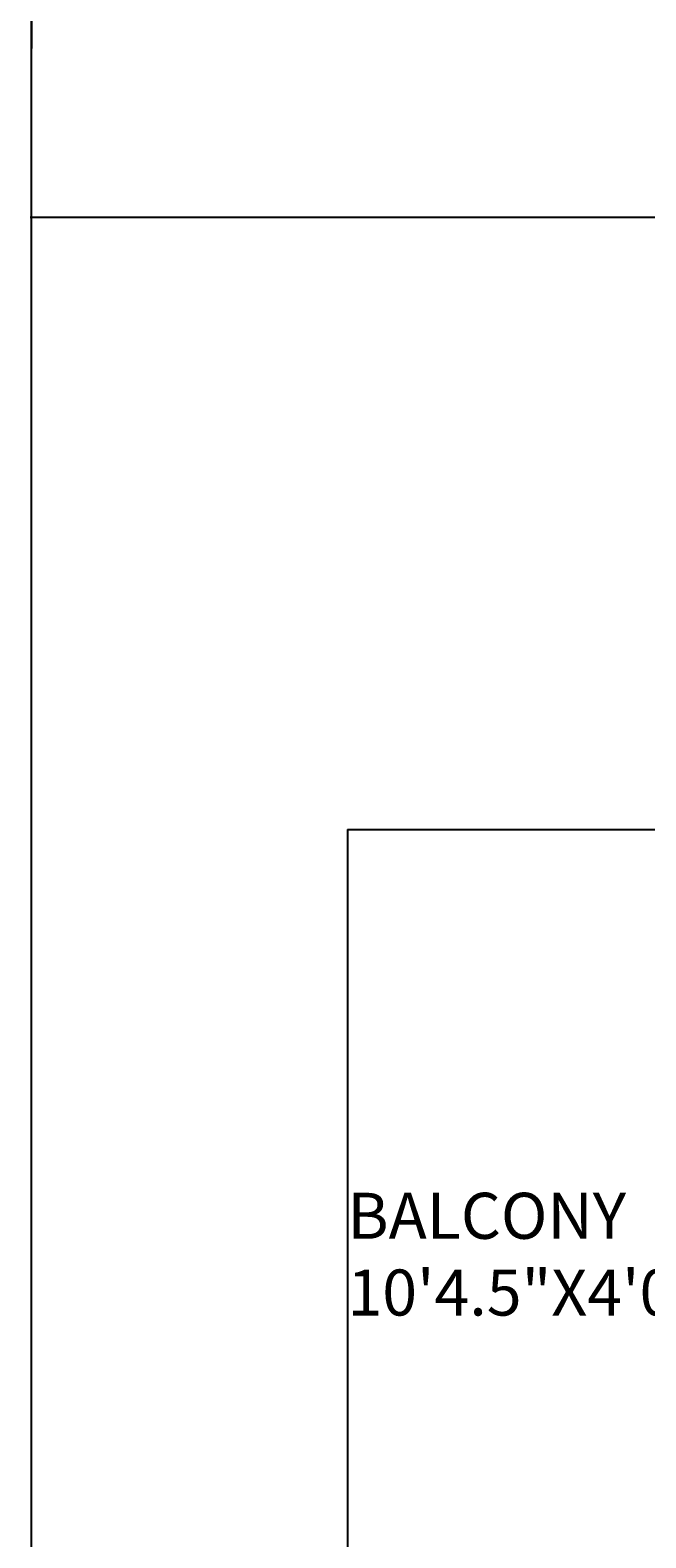
# Model space of a CAD drawing. Units: inches. Extents: x 2540 to 3167, y 3083 to 4007.
# Tile 3 of 15: x 2540 to 2634, y 3313 to 3542. Entities that reach past the tile are written whole.
import ezdxf

# ---------------------------------------------------------------- set-up
doc = ezdxf.new("R2010")
doc.units = ezdxf.units.IN
for name, color, linetype, lineweight in [('A-ANNO-DIMS', 2, 'Continuous', 18), ('A-AREA-IDEN', 7, 'Continuous', 18), ('A-FLOR-EDGE', 7, 'Continuous', 25)]:
    doc.layers.add(name, color=color, linetype=linetype, lineweight=lineweight)
doc.styles.get("Standard").update_dxf_attribs({"font": 'arial.ttf'})
doc.dimstyles.get("Standard").update_dxf_attribs({"dimtxt": 0.18, "dimasz": 0.18, "dimexe": 0.18, "dimexo": 0.0625, "dimgap": 0.09, "dimtad": 0, "dimtih": 1, "dimtoh": 1, "dimdec": 4, "dimzin": 0, "dimdsep": 46, "dimtxsty": 'Standard', "dimcen": 0.09, "dimadec": 0, "dimazin": 0, "dimtfac": 1, "dimtdec": 4, "dimtofl": 0, "dimtmove": 0, "dimatfit": 3, "dimfxl": 1, "dimtolj": 1, "dimtzin": 0, "dimarcsym": 0})

# ---------------------------------------------------------------- blocks, each defined once
blk = doc.blocks.new('*D44')
at = {"layer": 'A-ANNO-DIMS', "color": 0, "lineweight": -2, "transparency": 16777216}
for p, q in [((2771.45, 3964.71), (2540.23, 3964.71)), ((2540.41, 3964.53), (2540.41, 3545.4)), ((2540.41, 3125.89), (2540.41, 3545.03)), ((2810.45, 3125.71), (2540.23, 3125.71))]:
    blk.add_line(p, q, dxfattribs=at)
at = {"layer": 'A-ANNO-DIMS', "color": 0, "transparency": 16777216}
for points in [[(2540.38, 3964.53), (2540.44, 3964.53), (2540.41, 3964.71)], [(2540.38, 3125.89), (2540.44, 3125.89), (2540.41, 3125.71)]]:
    blk.add_solid(points, dxfattribs=at)
at = {"layer": 'Defpoints', "color": 0, "transparency": 16777216}
for p in [(2540.41, 3964.71), (2771.51, 3964.71), (2810.51, 3125.71)]:
    blk.add_point(p, dxfattribs=at)
at = {"layer": 'A-ANNO-DIMS', "color": 0, "transparency": 16777216, "insert": (2540.41, 3545.21), "char_height": 0.18, "attachment_point": 5}
blk.add_mtext('\\A1;839', dxfattribs=at)
blk = doc.blocks.new('*D57')
at = {"layer": 'A-ANNO-DIMS', "color": 0, "lineweight": -2, "transparency": 16777216}
for p, q in [((2810.45, 3564.71), (2540.23, 3564.71)), ((2540.41, 3564.53), (2540.41, 3539.4)), ((2540.41, 3513.89), (2540.41, 3539.03)), ((2810.45, 3513.71), (2540.23, 3513.71))]:
    blk.add_line(p, q, dxfattribs=at)
at = {"layer": 'A-ANNO-DIMS', "color": 0, "transparency": 16777216}
for points in [[(2540.38, 3564.53), (2540.44, 3564.53), (2540.41, 3564.71)], [(2540.38, 3513.89), (2540.44, 3513.89), (2540.41, 3513.71)]]:
    blk.add_solid(points, dxfattribs=at)
at = {"layer": 'Defpoints', "color": 0, "transparency": 16777216}
for p in [(2810.51, 3564.71), (2540.41, 3513.71), (2810.51, 3513.71)]:
    blk.add_point(p, dxfattribs=at)
at = {"layer": 'A-ANNO-DIMS', "color": 0, "transparency": 16777216, "insert": (2540.41, 3539.21), "char_height": 0.18, "attachment_point": 5}
blk.add_mtext('\\A1;51', dxfattribs=at)

msp = doc.modelspace()

# ---------------------------------------------------------------- linework, layer by layer
at = {"layer": 'A-FLOR-EDGE'}
for q in [(2636.51, 3420.71), (2588.51, 3290.71)]:
    msp.add_line((2588.51, 3420.71), q, dxfattribs=at)

# ---------------------------------------------------------------- texts
at = {"layer": 'A-AREA-IDEN', "insert": (2588.51, 3365.46), "char_height": 7, "attachment_point": 1}
msp.add_mtext_dynamic_manual_height_columns('BALCONY\\P10\'4.5"X4\'0"', width=97.3161, gutter_width=12.5, heights=[0], dxfattribs=at)

# ---------------------------------------------------------------- dimensions: what is measured, and where the dimension line sits
at = {"layer": 'A-ANNO-DIMS'}
for base, p1, p2, picture, middle in [((2540.41, 3964.71), (2810.51, 3125.71), (2771.51, 3964.71), '*D44', (2540.41, 3545.21)), ((2540.41, 3513.71), (2810.51, 3564.71), (2810.51, 3513.71), '*D57', (2540.41, 3539.21))]:
    dim = msp.add_linear_dim(base=base, p1=p1, p2=p2, angle=90, dimstyle='Standard', override={"dimdec": 0, "dimlfac": 1, "dimrnd": 0, "dimzin": 0, "dimdsep": 46, "dimlunit": 2}, dxfattribs=at)
    dim.commit()
    dim.dimension.update_dxf_attribs({"geometry": picture, "text_midpoint": middle})

doc.saveas('drawing.dxf')
